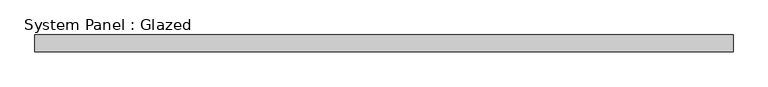
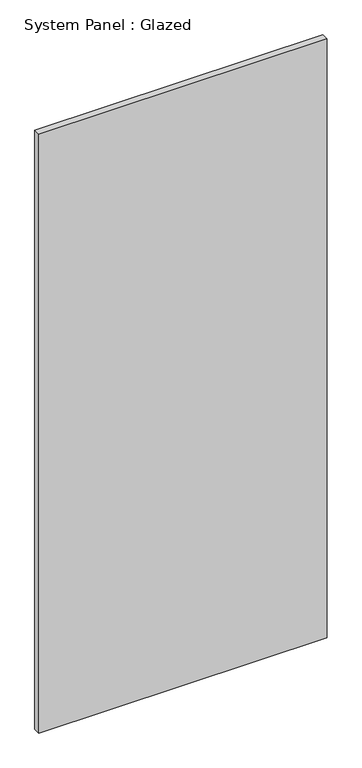
"""IFC4 building model written with IfcOpenShell, lengths in millimetres: plate geometry, System Panel : Glazed."""

from ifc_helpers import new_model, si_unit, origin, origin_with_axes, place, context, project, spatial, polyline, outline, extrude, source, transform, mapped, element, save


def system_panel_glazed_daed1646(model_context):
    return source(origin(), model_context, "Body", "SweptSolid", [
        extrude(outline(polyline([(533.4, 19.05), (-533.4, 19.05), (-533.4, 44.45), (533.4, 44.45), (533.4, 19.05)])), origin_with_axes(), (0.0, 0.0, 1.0), 2343.15),
    ])


if __name__ == "__main__":
    model = new_model("IFC4")
    model_context = context("Model", 3, world=origin())
    ifc_project = project(units=[si_unit("LENGTHUNIT", "METRE", prefix="MILLI")], contexts=[model_context])
    site = spatial("IfcSite", under=ifc_project)
    building = spatial("IfcBuilding", under=site)
    placement = place(None, origin())
    system_panel_glazed_shape = system_panel_glazed_daed1646(model_context)
    element("IfcPlate", 1, ObjectType="System Panel : Glazed", at=placement, inside=building, context=model_context, shape_type="MappedRepresentation", body=[
        mapped(system_panel_glazed_shape, transform((0.0, 0.0, 0.0), x_axis=(1.0, 0.0, 0.0), y_axis=(0.0, 1.0, 0.0), z_axis=(0.0, 0.0, 1.0))),
    ])
    save(model, "model.ifc")

# Revit data of these elements
# Type "System Panel : Glazed"
#   Construction Type Id = "GSP4R"
#   Analytic Construction = "1/8 in Pilkington single glazing"
#   Visual Light Transmittance = 0.9
#   Solar Heat Gain Coefficient = 0.86
#   Heat Transfer Coefficient (U) = 1.18115 BTU/(h·ft²·°F)
#   Define Thermal Properties by = 1
# Element 1 (IfcPlate, "System Panel : Glazed")
#   Materials on its faces: "Glass"
# Materials
#   "Glass": class "Glass", colour RGB 0 128 192, transparency 0.75, Description = "Soda Lime Glass", Cost = 0
